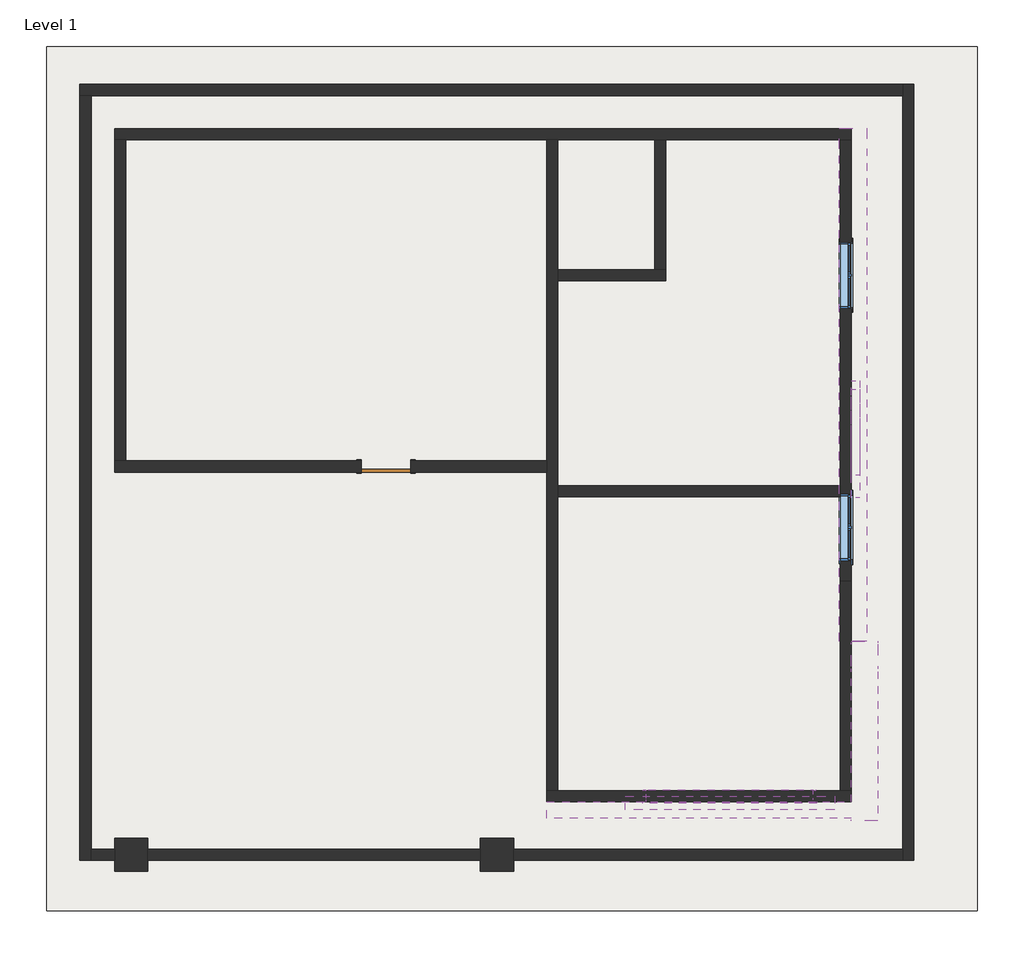
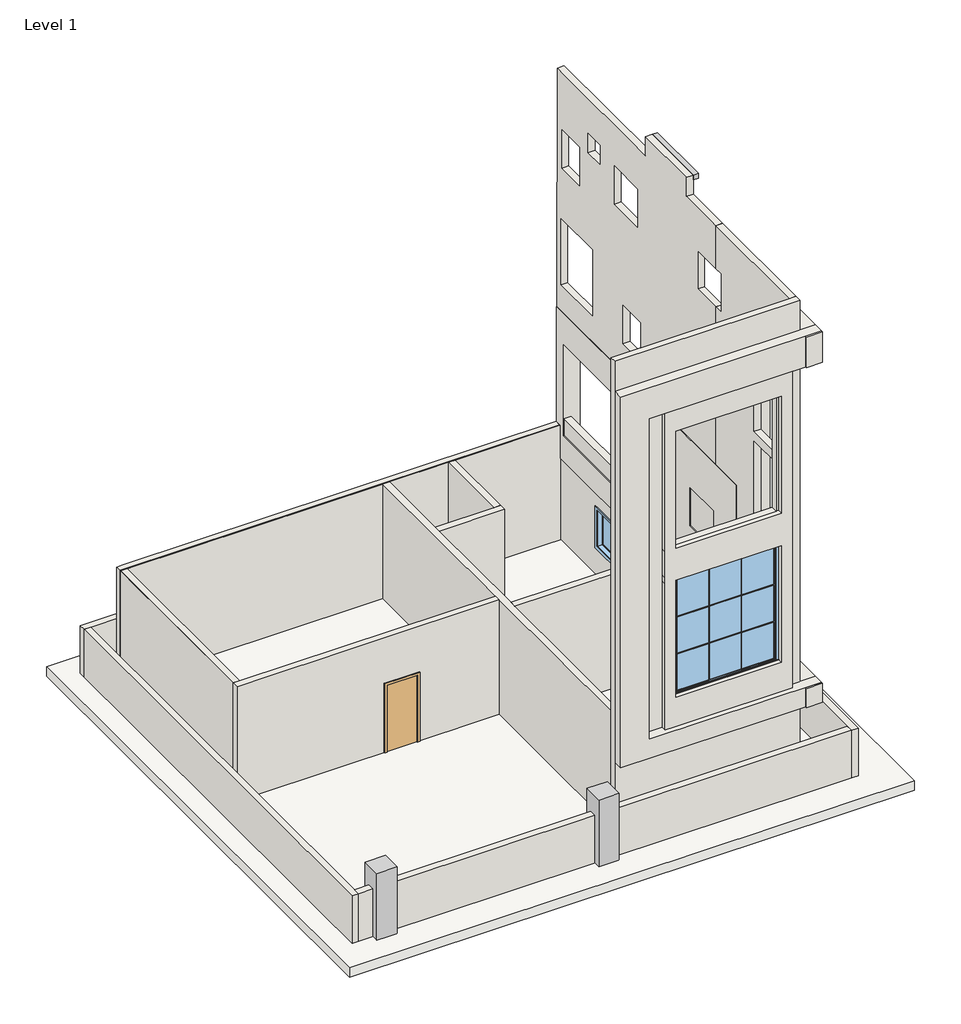
# One storey: 19 walls, 3 windows, 2 columns, 2 proxies, 1 door, 1 slab.
"""IFC4 building model written with IfcOpenShell, lengths in millimetres."""

from ifc_helpers import new_model, si_unit, frame, origin, origin_with_axes, place, context, project, spatial, polyline, outline, extrude, faceted_brep, transform, mapped, element, save
from components import door_54dd4da4, walls_1_walls_1_fa617820, walls_5_walls_5_f65b2cef, walls_7_walls_7_b227ebcc, window_cae7f124, window_0862ab64

model = new_model("IFC4")

# Units and contexts
model_context = context("Model", 3, world=origin())
ifc_project = project(units=[si_unit("LENGTHUNIT", "METRE", prefix="MILLI")], contexts=[model_context])

# Site, building, storey
site = spatial("IfcSite", under=ifc_project)
building = spatial("IfcBuilding", under=site)
storey = spatial("IfcBuildingStorey", under=building, Name="Level 1", Elevation=0.0)

# Proxies
placement = place(None, origin())
element("IfcBuildingElementProxy", 1, Name="Cornice", ObjectType="Cornice", at=placement, inside=storey, context=model_context, shape_type="SweptSolid", body=[
    extrude(outline(polyline([(1662.3254876, 6733.2171591), (1814.7254876, 6733.2171591), (1814.7254876, 4588.9609482), (1662.3254876, 4588.9609482), (1662.3254876, 6733.2171591)])), frame((0.0, 0.0, 15392.4), z_axis=(0.0, 0.0, 1.0), x_axis=(1.0, 0.0, 0.0)), (0.0, 0.0, 1.0), 152.4),
])
element("IfcBuildingElementProxy", 2, Name="Cornice", ObjectType="Cornice", at=placement, inside=storey, context=model_context, shape_type="SweptSolid", body=[
    extrude(outline(polyline([(1662.3254876, 6572.7173646), (1814.7254876, 6572.7173646), (1814.7254876, 4997.9173646), (1662.3254876, 4997.9173646), (1662.3254876, 6572.7173646)])), frame((0.0, 0.0, 12192.0), z_axis=(0.0, 0.0, 1.0), x_axis=(1.0, 0.0, 0.0)), (0.0, 0.0, 1.0), 152.4),
])

# Columns
element("IfcColumn", 3, ObjectType="Rectangular Column : 24\" x 24\"", at=placement, inside=storey, context=model_context, shape_type="Brep", body=[
    faceted_brep([(-11240.8745124, -1652.1419198, 2133.6), (-11850.4745124, -1652.1419198, 2133.6), (-11850.4745124, -2261.7419198, 2133.6), (-11240.8745124, -2261.7419198, 2133.6), (-11240.8745124, -1652.1419198, 0.0), (-11240.8745124, -1855.3419198, 0.0), (-11240.8745124, -2058.5419198, 0.0), (-11240.8745124, -2261.7419198, 0.0), (-11850.4745124, -2261.7419198, 0.0), (-11850.4745124, -2058.5419198, 0.0), (-11850.4745124, -1855.3419198, 0.0), (-11850.4745124, -1652.1419198, 0.0)], [[[0, 1, 2, 3]], [[4, 5, 6, 7, 8, 9, 10, 11]], [[1, 0, 4, 11]], [[2, 1, 11, 10, 9, 8]], [[3, 2, 8, 7]], [[0, 3, 7, 6, 5, 4]]]),
])
element("IfcColumn", 4, ObjectType="Rectangular Column : 24\" x 24\"", at=placement, inside=storey, context=model_context, shape_type="Brep", body=[
    faceted_brep([(-4533.4058988, -1652.1419198, 2133.6), (-5143.0058988, -1652.1419198, 2133.6), (-5143.0058988, -2261.7419198, 2133.6), (-4533.4058988, -2261.7419198, 2133.6), (-4533.4058988, -1652.1419198, 0.0), (-4533.4058988, -1855.3419198, 0.0), (-4533.4058988, -2058.5419198, 0.0), (-4533.4058988, -2261.7419198, 0.0), (-5143.0058988, -2261.7419198, 0.0), (-5143.0058988, -2058.5419198, 0.0), (-5143.0058988, -1855.3419198, 0.0), (-5143.0058988, -1652.1419198, 0.0)], [[[0, 1, 2, 3]], [[4, 5, 6, 7, 8, 9, 10, 11]], [[1, 0, 4, 11]], [[2, 1, 11, 10, 9, 8]], [[3, 2, 8, 7]], [[0, 3, 7, 6, 5, 4]]]),
])

# Door
door_shape = door_54dd4da4(model_context)
element("IfcDoor", 5, ObjectType="Single-Flush : 36\" x 84\"", at=placement, inside=storey, context=model_context, shape_type="MappedRepresentation", body=[
    mapped(door_shape, transform((-6872.0745124, 5160.4609482, 0.0), x_axis=(-1.0, 0.0, 0.0), y_axis=(0.0, -1.0, 0.0), z_axis=(0.0, 0.0, 1.0))),
])

# Slab
element("IfcSlab", 6, ObjectType="Generic - 12\"", at=placement, inside=storey, context=model_context, shape_type="SweptSolid", body=[
    extrude(outline(polyline([(3972.1194136, 12860.9919886), (3972.1194136, -2988.6080114), (-13096.6805864, -2988.6080114), (-13096.6805864, 12860.9919886), (3972.1194136, 12860.9919886)])), frame((0.0, 0.0, -304.8), z_axis=(0.0, 0.0, 1.0), x_axis=(1.0, 0.0, 0.0)), (0.0, 0.0, 1.0), 304.8),
])

# Walls
element("IfcWall", 7, ObjectType="Generic - 8\"", at=placement, inside=storey, context=model_context, shape_type="Brep", body=[
    faceted_brep([(-11850.4745124, 11154.8609482, 0.0), (-11647.2745124, 11154.8609482, 0.0), (-3925.6745124, 11154.8609482, 0.0), (-3722.4745124, 11154.8609482, 0.0), (-1944.4745124, 11154.8609482, 0.0), (-1741.2745124, 11154.8609482, 0.0), (1459.1254876, 11154.8609482, 0.0), (1662.3254876, 11154.8609482, 0.0), (1662.3254876, 11154.8609482, 3657.6), (1459.1254876, 11154.8609482, 3657.6), (1433.7254876, 11154.8609482, 3657.6), (-1741.2745124, 11154.8609482, 3657.6), (-1944.4745124, 11154.8609482, 3657.6), (-3722.4745124, 11154.8609482, 3657.6), (-3925.6745124, 11154.8609482, 3657.6), (-11647.2745124, 11154.8609482, 3657.6), (-11847.2995124, 11154.8609482, 3657.6), (-11850.4745124, 11154.8609482, 3657.6), (-11850.4745124, 11358.0609482, 0.0), (-11850.4745124, 11358.0609482, 3657.6), (-11847.2995124, 11358.0609482, 3657.6), (-11647.2745124, 11358.0609482, 3657.6), (1433.7254876, 11358.0609482, 3657.6), (1459.1254876, 11358.0609482, 3657.6), (1662.3254876, 11358.0609482, 3657.6), (1662.3254876, 11358.0609482, 0.0), (1662.3254876, 11192.9609482, 3657.6), (-11850.4745124, 11192.9609482, 3657.6), (1433.7254876, 11192.9609482, 3657.6), (-11847.2995124, 11192.9609482, 3657.6)], [[[0, 1, 2, 3, 4, 5, 6, 7, 8, 9, 10, 11, 12, 13, 14, 15, 16, 17]], [[18, 19, 20, 21, 22, 23, 24, 25]], [[7, 6, 5, 4, 3, 2, 1, 0, 18, 25]], [[8, 7, 25, 24, 26]], [[0, 17, 27, 19, 18]], [[10, 9, 8, 26, 28]], [[26, 24, 23, 22, 28]], [[17, 16, 29, 27]], [[22, 21, 20, 29, 28]], [[20, 19, 27, 29]], [[16, 15, 14, 13, 12, 11, 10, 28, 29]]]),
])
element("IfcWall", 8, ObjectType="Generic - 8\"", at=placement, inside=storey, context=model_context, shape_type="Brep", body=[
    faceted_brep([(-11850.4745124, 5058.8609482, 0.0), (-7329.2745124, 5058.8609482, 0.0), (-7329.2745124, 5058.8609482, 2133.6), (-6414.8745124, 5058.8609482, 2133.6), (-6414.8745124, 5058.8609482, 0.0), (-3925.6745124, 5058.8609482, 0.0), (-3925.6745124, 5058.8609482, 3657.6), (-11847.2995124, 5058.8609482, 3657.6), (-11850.4745124, 5058.8609482, 3657.6), (-7329.2745124, 5262.0609482, 2133.6), (-7329.2745124, 5262.0609482, 0.0), (-11647.2745124, 5262.0609482, 0.0), (-11850.4745124, 5262.0609482, 0.0), (-11850.4745124, 5262.0609482, 3657.6), (-11847.2995124, 5262.0609482, 3657.6), (-11647.2745124, 5262.0609482, 3657.6), (-3925.6745124, 5262.0609482, 3657.6), (-3925.6745124, 5262.0609482, 0.0), (-6414.8745124, 5262.0609482, 0.0), (-6414.8745124, 5262.0609482, 2133.6)], [[[0, 1, 2, 3, 4, 5, 6, 7, 8]], [[9, 10, 11, 12, 13, 14, 15, 16, 17, 18, 19]], [[18, 17, 5, 4]], [[12, 11, 10, 1, 0]], [[6, 5, 17, 16]], [[0, 8, 13, 12]], [[8, 7, 14, 13]], [[7, 6, 16, 15, 14]], [[2, 1, 10, 9]], [[3, 2, 9, 19]], [[4, 3, 19, 18]]]),
])
element("IfcWall", 9, ObjectType="Generic - 8\"", at=placement, inside=storey, context=model_context, shape_type="Brep", body=[
    faceted_brep([(-3925.6745124, 11154.8609482, 0.0), (-3925.6745124, 5262.0609482, 0.0), (-3925.6745124, 5058.8609482, 0.0), (-3925.6745124, -783.1390518, 0.0), (-3925.6745124, -783.1390518, 3657.6), (-3925.6745124, 1858.4609482, 3657.6), (-3925.6745124, 5058.8609482, 3657.6), (-3925.6745124, 5262.0609482, 3657.6), (-3925.6745124, 11154.8609482, 3657.6), (-3722.4745124, 11154.8609482, 0.0), (-3722.4745124, 11154.8609482, 3657.6), (-3722.4745124, 8767.2609482, 3657.6), (-3722.4745124, 8564.0609482, 3657.6), (-3722.4745124, 4804.8609482, 3657.6), (-3722.4745124, 4601.6609482, 3657.6), (-3722.4745124, 1858.4609482, 3657.6), (-3722.4745124, -783.1390518, 3657.6), (-3722.4745124, -783.1390518, 0.0), (-3722.4745124, 4601.6609482, 0.0), (-3722.4745124, 4804.8609482, 0.0), (-3722.4745124, 8564.0609482, 0.0), (-3722.4745124, 8767.2609482, 0.0)], [[[0, 1, 2, 3, 4, 5, 6, 7, 8]], [[9, 10, 11, 12, 13, 14, 15, 16, 17, 18, 19, 20, 21]], [[3, 2, 1, 0, 9, 21, 20, 19, 18, 17]], [[8, 7, 6, 5, 4, 16, 15, 14, 13, 12, 11, 10]], [[4, 3, 17, 16]], [[0, 8, 10, 9]]]),
])
element("IfcWall", 10, ObjectType="Generic - 8\"", at=placement, inside=storey, context=model_context, shape_type="SweptSolid", body=[
    extrude(outline(polyline([(3657.6, -11850.4745124), (0.0, -11850.4745124), (0.0, -11647.2745124), (3657.6, -11647.2745124), (3657.6, -11847.2995124), (3657.6, -11850.4745124)])), frame((0.0, 5262.0609482, 0.0), z_axis=(0.0, 1.0, 0.0), x_axis=(0.0, 0.0, 1.0)), (0.0, 0.0, 1.0), 5892.8),
])
element("IfcWall", 11, ObjectType="Generic - 8\"", at=placement, inside=storey, context=model_context, shape_type="Brep", body=[
    faceted_brep([(-3925.6745124, -986.3390518, 14935.2), (-3925.6745124, -986.3390518, 0.0), (1662.3254876, -986.3390518, 0.0), (1662.3254876, -986.3390518, 14935.2), (-2096.8745124, -986.3390518, 12107.4316285), (951.1254876, -986.3390518, 12107.4316285), (951.1254876, -986.3390518, 8449.8316285), (-2096.8745124, -986.3390518, 8449.8316285), (-2096.8745124, -986.3390518, 7347.484706), (951.1254876, -986.3390518, 7347.484706), (951.1254876, -986.3390518, 3689.884706), (-2096.8745124, -986.3390518, 3689.884706), (-3925.6745124, -783.1390518, 0.0), (-3925.6745124, -783.1390518, 3657.6), (-3925.6745124, -783.1390518, 10972.8), (-3925.6745124, -783.1390518, 14935.2), (1459.1254876, -783.1390518, 14935.2), (1662.3254876, -783.1390518, 14935.2), (1662.3254876, -783.1390518, 0.0), (1459.1254876, -783.1390518, 0.0), (-3722.4745124, -783.1390518, 0.0), (-2096.8745124, -783.1390518, 12107.4316285), (-2096.8745124, -783.1390518, 8449.8316285), (951.1254876, -783.1390518, 8449.8316285), (951.1254876, -783.1390518, 12107.4316285), (-2096.8745124, -783.1390518, 7347.484706), (-2096.8745124, -783.1390518, 3689.884706), (951.1254876, -783.1390518, 3689.884706), (951.1254876, -783.1390518, 7347.484706)], [[[0, 1, 2, 3], [4, 5, 6, 7], [8, 9, 10, 11]], [[12, 13, 14, 15, 16, 17, 18, 19, 20], [21, 22, 23, 24], [25, 26, 27, 28]], [[2, 1, 12, 20, 19, 18]], [[0, 3, 17, 16, 15]], [[3, 2, 18, 17]], [[0, 15, 14, 13, 12, 1]], [[22, 21, 4, 7]], [[23, 22, 7, 6]], [[24, 23, 6, 5]], [[21, 24, 5, 4]], [[26, 25, 8, 11]], [[27, 26, 11, 10]], [[28, 27, 10, 9]], [[25, 28, 9, 8]]]),
])
element("IfcWall", 12, ObjectType="Generic - 8\"", at=placement, inside=storey, context=model_context, shape_type="SweptSolid", body=[
    extrude(outline(polyline([(3052.2609482, 0.0), (-783.1390518, 0.0), (-783.1390518, 14935.2), (3052.2609482, 14935.2), (3052.2609482, 13563.6), (2772.8609482, 13563.6), (2772.8609482, 12344.4), (3052.2609482, 12344.4), (3052.2609482, 0.0)]), holes=[polyline([(1055.2332725, 9576.1019988), (1055.2332725, 12522.5019988), (-163.9667275, 12522.5019988), (-163.9667275, 9576.1019988), (1055.2332725, 9576.1019988)]), polyline([(1055.2332725, 6324.9019988), (1055.2332725, 9271.3019988), (-163.9667275, 9271.3019988), (-163.9667275, 6324.9019988), (1055.2332725, 6324.9019988)]), polyline([(1055.2332725, 3022.9019988), (1055.2332725, 5969.3019988), (-163.9667275, 5969.3019988), (-163.9667275, 3022.9019988), (1055.2332725, 3022.9019988)])]), frame((1459.1254876, 0.0, 0.0), z_axis=(1.0, 0.0, 0.0), x_axis=(0.0, 1.0, 0.0)), (0.0, 0.0, 1.0), 203.2),
])
element("IfcWall", 13, ObjectType="Generic - 8\"", at=placement, inside=storey, context=model_context, shape_type="Brep", body=[
    faceted_brep([(1459.1254876, 11154.8609482, 0.0), (1459.1254876, 4804.8609482, 0.0), (1459.1254876, 4601.6609482, 0.0), (1459.1254876, 3052.2609482, 0.0), (1459.1254876, 3052.2609482, 12344.4), (1459.1254876, 3992.0609482, 12344.4), (1459.1254876, 3992.0609482, 13563.6), (1459.1254876, 3052.2609482, 13563.6), (1459.1254876, 3052.2609482, 14935.2), (1459.1254876, 4588.9609482, 14935.2), (1459.1254876, 4588.9609482, 15544.8), (1459.1254876, 6733.2171591, 15544.8), (1459.1254876, 6733.2171591, 14935.2), (1459.1254876, 11142.1609482, 14935.2), (1459.1254876, 11345.3609482, 14935.2), (1459.1254876, 11345.3609482, 11277.6), (1459.1254876, 11358.0609482, 11277.6), (1459.1254876, 11358.0609482, 7623.0321664), (1459.1254876, 11358.0609482, 7315.2), (1459.1254876, 11358.0609482, 3657.6), (1459.1254876, 11154.8609482, 3657.6), (1459.1254876, 9732.4609482, 13828.4684583), (1459.1254876, 9122.8609482, 13828.4684583), (1459.1254876, 9122.8609482, 13218.8684583), (1459.1254876, 9732.4609482, 13218.8684583), (1459.1254876, 7141.6609482, 13622.4204192), (1459.1254876, 7141.6609482, 12403.2204192), (1459.1254876, 8360.8609482, 12403.2204192), (1459.1254876, 8360.8609482, 13622.4204192), (1459.1254876, 10189.6609482, 13106.4), (1459.1254876, 10189.6609482, 11887.2), (1459.1254876, 11104.0609482, 11887.2), (1459.1254876, 11104.0609482, 13106.4), (1459.1254876, 4855.6609482, 9448.8), (1459.1254876, 3941.2609482, 9448.8), (1459.1254876, 3941.2609482, 8229.6), (1459.1254876, 4855.6609482, 8229.6), (1459.1254876, 7903.6609482, 9448.8), (1459.1254876, 6989.2609482, 9448.8), (1459.1254876, 6989.2609482, 8229.6), (1459.1254876, 7903.6609482, 8229.6), (1459.1254876, 11154.8609482, 10244.4876686), (1459.1254876, 9518.25414, 10244.4876686), (1459.1254876, 9518.25414, 8130.9177257), (1459.1254876, 11154.8609482, 8130.9177257), (1459.1254876, 3433.2609482, 2133.6), (1459.1254876, 3433.2609482, 914.4), (1459.1254876, 4652.4609482, 914.4), (1459.1254876, 4652.4609482, 2133.6), (1459.1254876, 8056.0609482, 2133.6), (1459.1254876, 8056.0609482, 914.4), (1459.1254876, 9275.2609482, 914.4), (1459.1254876, 9275.2609482, 2133.6), (1459.1254876, 10990.2518123, 6324.9019988), (1459.1254876, 7724.717248, 6324.9019988), (1459.1254876, 7724.717248, 3962.4), (1459.1254876, 10990.2518123, 3962.4), (1459.1254876, 7185.0917513, 6324.9019988), (1459.1254876, 5580.0518123, 6324.9019988), (1459.1254876, 5580.0518123, 3962.4), (1459.1254876, 7185.0917513, 3962.4), (1662.3254876, 3052.2609482, 0.0), (1662.3254876, 11154.8609482, 0.0), (1662.3254876, 11154.8609482, 3657.6), (1662.3254876, 11358.0609482, 3657.6), (1662.3254876, 11358.0609482, 11277.6), (1662.3254876, 11345.3609482, 11277.6), (1662.3254876, 11345.3609482, 14935.2), (1662.3254876, 6733.2171591, 14935.2), (1662.3254876, 6733.2171591, 15544.8), (1662.3254876, 4588.9609482, 15544.8), (1662.3254876, 4588.9609482, 14935.2), (1662.3254876, 3052.2609482, 14935.2), (1662.3254876, 3052.2609482, 13563.6), (1662.3254876, 3992.0609482, 13563.6), (1662.3254876, 3992.0609482, 12344.4), (1662.3254876, 3052.2609482, 12344.4), (1662.3254876, 9732.4609482, 13828.4684583), (1662.3254876, 9732.4609482, 13218.8684583), (1662.3254876, 9122.8609482, 13218.8684583), (1662.3254876, 9122.8609482, 13828.4684583), (1662.3254876, 7141.6609482, 13622.4204192), (1662.3254876, 8360.8609482, 13622.4204192), (1662.3254876, 8360.8609482, 12403.2204192), (1662.3254876, 7141.6609482, 12403.2204192), (1662.3254876, 10189.6609482, 13106.4), (1662.3254876, 11104.0609482, 13106.4), (1662.3254876, 11104.0609482, 11887.2), (1662.3254876, 10189.6609482, 11887.2), (1662.3254876, 4855.6609482, 9448.8), (1662.3254876, 4855.6609482, 8229.6), (1662.3254876, 3941.2609482, 8229.6), (1662.3254876, 3941.2609482, 9448.8), (1662.3254876, 7903.6609482, 9448.8), (1662.3254876, 7903.6609482, 8229.6), (1662.3254876, 6989.2609482, 8229.6), (1662.3254876, 6989.2609482, 9448.8), (1662.3254876, 9518.25414, 10244.4876686), (1662.3254876, 11154.8609482, 10244.4876686), (1662.3254876, 11154.8609482, 8130.9177257), (1662.3254876, 9518.25414, 8130.9177257), (1662.3254876, 3433.2609482, 2133.6), (1662.3254876, 4652.4609482, 2133.6), (1662.3254876, 4652.4609482, 914.4), (1662.3254876, 3433.2609482, 914.4), (1662.3254876, 8056.0609482, 2133.6), (1662.3254876, 9275.2609482, 2133.6), (1662.3254876, 9275.2609482, 914.4), (1662.3254876, 8056.0609482, 914.4), (1662.3254876, 7724.717248, 6324.9019988), (1662.3254876, 10990.2518123, 6324.9019988), (1662.3254876, 10990.2518123, 3962.4), (1662.3254876, 7724.717248, 3962.4), (1662.3254876, 5580.0518123, 6324.9019988), (1662.3254876, 7185.0917513, 6324.9019988), (1662.3254876, 7185.0917513, 3962.4), (1662.3254876, 5580.0518123, 3962.4)], [[[0, 1, 2, 3, 4, 5, 6, 7, 8, 9, 10, 11, 12, 13, 14, 15, 16, 17, 18, 19, 20], [21, 22, 23, 24], [25, 26, 27, 28], [29, 30, 31, 32], [33, 34, 35, 36], [37, 38, 39, 40], [41, 42, 43, 44], [45, 46, 47, 48], [49, 50, 51, 52], [53, 54, 55, 56], [57, 58, 59, 60]], [[61, 62, 63, 64, 65, 66, 67, 68, 69, 70, 71, 72, 73, 74, 75, 76], [77, 78, 79, 80], [81, 82, 83, 84], [85, 86, 87, 88], [89, 90, 91, 92], [93, 94, 95, 96], [97, 98, 99, 100], [101, 102, 103, 104], [105, 106, 107, 108], [109, 110, 111, 112], [113, 114, 115, 116]], [[0, 20, 63, 62]], [[19, 18, 17, 16, 65, 64]], [[15, 14, 67, 66]], [[3, 2, 1, 0, 62, 61]], [[3, 61, 76, 4]], [[72, 8, 7, 73]], [[64, 63, 20, 19]], [[66, 65, 16, 15]], [[9, 8, 72, 71]], [[10, 9, 71, 70]], [[11, 10, 70, 69]], [[12, 11, 69, 68]], [[14, 13, 12, 68, 67]], [[78, 77, 21, 24]], [[79, 78, 24, 23]], [[80, 79, 23, 22]], [[77, 80, 22, 21]], [[75, 5, 4, 76]], [[5, 75, 74, 6]], [[6, 74, 73, 7]], [[26, 25, 81, 84]], [[27, 26, 84, 83]], [[28, 27, 83, 82]], [[25, 28, 82, 81]], [[30, 29, 85, 88]], [[31, 30, 88, 87]], [[32, 31, 87, 86]], [[29, 32, 86, 85]], [[90, 89, 33, 36]], [[91, 90, 36, 35]], [[92, 91, 35, 34]], [[89, 92, 34, 33]], [[94, 93, 37, 40]], [[95, 94, 40, 39]], [[96, 95, 39, 38]], [[93, 96, 38, 37]], [[42, 41, 98, 97]], [[43, 42, 97, 100]], [[44, 43, 100, 99]], [[41, 44, 99, 98]], [[46, 45, 101, 104]], [[47, 46, 104, 103]], [[48, 47, 103, 102]], [[45, 48, 102, 101]], [[50, 49, 105, 108]], [[51, 50, 108, 107]], [[52, 51, 107, 106]], [[49, 52, 106, 105]], [[54, 53, 110, 109]], [[55, 54, 109, 112]], [[56, 55, 112, 111]], [[53, 56, 111, 110]], [[58, 57, 114, 113]], [[59, 58, 113, 116]], [[60, 59, 116, 115]], [[57, 60, 115, 114]]]),
])
element("IfcWall", 14, ObjectType="Generic - 8\"", at=placement, inside=storey, context=model_context, shape_type="SweptSolid", body=[
    extrude(outline(polyline([(1459.1254876, 4601.6609482), (-3722.4745124, 4601.6609482), (-3722.4745124, 4804.8609482), (1459.1254876, 4804.8609482), (1459.1254876, 4601.6609482)])), origin_with_axes(), (0.0, 0.0, 1.0), 3657.6),
])
element("IfcWall", 15, ObjectType="Generic - 8\"", at=placement, inside=storey, context=model_context, shape_type="Brep", body=[
    faceted_brep([(-3722.4745124, 8564.0609482, 0.0), (-1741.2745124, 8564.0609482, 0.0), (-1741.2745124, 8564.0609482, 3657.6), (-3722.4745124, 8564.0609482, 3657.6), (-3722.4745124, 8767.2609482, 0.0), (-3722.4745124, 8767.2609482, 3657.6), (-1944.4745124, 8767.2609482, 3657.6), (-1741.2745124, 8767.2609482, 3657.6), (-1741.2745124, 8767.2609482, 0.0), (-1944.4745124, 8767.2609482, 0.0)], [[[0, 1, 2, 3]], [[4, 5, 6, 7, 8, 9]], [[1, 0, 4, 9, 8]], [[3, 2, 7, 6, 5]], [[0, 3, 5, 4]], [[2, 1, 8, 7]]]),
])
element("IfcWall", 16, ObjectType="Generic - 8\"", at=placement, inside=storey, context=model_context, shape_type="SweptSolid", body=[
    extrude(outline(polyline([(-1741.2745124, 11154.8609482), (-1741.2745124, 8767.2609482), (-1944.4745124, 8767.2609482), (-1944.4745124, 11154.8609482), (-1741.2745124, 11154.8609482)])), origin_with_axes(), (0.0, 0.0, 1.0), 3657.6),
])
element("IfcWall", 17, ObjectType="Generic - 8\"", at=placement, inside=storey, context=model_context, shape_type="Brep", body=[
    faceted_brep([(-12483.6058988, 11962.2580802, 0.0), (-12280.4058988, 11962.2580802, 0.0), (2603.9941012, 11962.2580802, 0.0), (2603.9941012, 11962.2580802, 1524.0), (-12280.4058988, 11962.2580802, 1524.0), (-12483.6058988, 11962.2580802, 1524.0), (-12483.6058988, 12165.4580802, 0.0), (-12483.6058988, 12165.4580802, 1524.0), (2603.9941012, 12165.4580802, 1524.0), (2603.9941012, 12165.4580802, 0.0)], [[[0, 1, 2, 3, 4, 5]], [[6, 7, 8, 9]], [[2, 1, 0, 6, 9]], [[5, 4, 3, 8, 7]], [[0, 5, 7, 6]], [[3, 2, 9, 8]]]),
])
element("IfcWall", 18, ObjectType="Generic - 8\"", at=placement, inside=storey, context=model_context, shape_type="Brep", body=[
    faceted_brep([(-12280.4058988, -2058.5419198, 0.0), (-12280.4058988, -1855.3419198, 0.0), (-12280.4058988, 11962.2580802, 0.0), (-12280.4058988, 11962.2580802, 1524.0), (-12280.4058988, -1855.3419198, 1524.0), (-12280.4058988, -2058.5419198, 1524.0), (-12483.6058988, -2058.5419198, 0.0), (-12483.6058988, -2058.5419198, 1524.0), (-12483.6058988, 11962.2580802, 1524.0), (-12483.6058988, 11962.2580802, 0.0)], [[[0, 1, 2, 3, 4, 5]], [[6, 7, 8, 9]], [[2, 1, 0, 6, 9]], [[5, 4, 3, 8, 7]], [[3, 2, 9, 8]], [[0, 5, 7, 6]]]),
])
element("IfcWall", 19, ObjectType="Generic - 8\"", at=placement, inside=storey, context=model_context, shape_type="SweptSolid", body=[
    extrude(outline(polyline([(-11240.8745124, -1855.3419198), (-5143.0058988, -1855.3419198), (-5143.0058988, -2058.5419198), (-11240.8745124, -2058.5419198), (-11240.8745124, -1855.3419198)])), origin_with_axes(), (0.0, 0.0, 1.0), 1524.0),
])
element("IfcWall", 20, ObjectType="Generic - 8\"", at=placement, inside=storey, context=model_context, shape_type="Brep", body=[
    faceted_brep([(2603.9941012, 12165.4580802, 0.0), (2603.9941012, 11962.2580802, 0.0), (2603.9941012, -1855.3419198, 0.0), (2603.9941012, -2058.5419198, 0.0), (2603.9941012, -2058.5419198, 1524.0), (2603.9941012, -1855.3419198, 1524.0), (2603.9941012, 11962.2580802, 1524.0), (2603.9941012, 12165.4580802, 1524.0), (2807.1941012, 12165.4580802, 0.0), (2807.1941012, 12165.4580802, 1524.0), (2807.1941012, -2058.5419198, 1524.0), (2807.1941012, -2058.5419198, 0.0)], [[[0, 1, 2, 3, 4, 5, 6, 7]], [[8, 9, 10, 11]], [[3, 2, 1, 0, 8, 11]], [[7, 6, 5, 4, 10, 9]], [[0, 7, 9, 8]], [[4, 3, 11, 10]]]),
])
element("IfcWall", 21, ObjectType="Generic - 8\"", at=placement, inside=storey, context=model_context, shape_type="SweptSolid", body=[
    extrude(outline(polyline([(-11850.4745124, -2058.5419198), (-12280.4058988, -2058.5419198), (-12280.4058988, -1855.3419198), (-11850.4745124, -1855.3419198), (-11850.4745124, -2058.5419198)])), origin_with_axes(), (0.0, 0.0, 1.0), 1524.0),
])
element("IfcWall", 22, ObjectType="Generic - 8\"", at=placement, inside=storey, context=model_context, shape_type="SweptSolid", body=[
    extrude(outline(polyline([(2603.9941012, -2058.5419198), (-4533.4058988, -2058.5419198), (-4533.4058988, -1855.3419198), (2603.9941012, -1855.3419198), (2603.9941012, -2058.5419198)])), origin_with_axes(), (0.0, 0.0, 1.0), 1524.0),
])
walls_1_walls_1_shape = walls_1_walls_1_fa617820(model_context)
element("IfcWall", 23, ObjectType="Walls 1 : Walls 1", at=placement, inside=storey, context=model_context, shape_type="MappedRepresentation", body=[
    mapped(walls_1_walls_1_shape, transform((0.0, 0.0, 0.0), x_axis=(1.0, 0.0, 0.0), y_axis=(0.0, 1.0, 0.0), z_axis=(0.0, 0.0, 1.0))),
])
walls_5_walls_5_shape = walls_5_walls_5_f65b2cef(model_context)
element("IfcWall", 24, ObjectType="Walls 5 : Walls 5", at=placement, inside=storey, context=model_context, shape_type="MappedRepresentation", body=[
    mapped(walls_5_walls_5_shape, transform((0.0, 0.0, 0.0), x_axis=(1.0, 0.0, 0.0), y_axis=(0.0, 1.0, 0.0), z_axis=(0.0, 0.0, 1.0))),
])
walls_7_walls_7_shape = walls_7_walls_7_b227ebcc(model_context)
element("IfcWall", 25, ObjectType="Walls 7 : Walls 7", at=placement, inside=storey, context=model_context, shape_type="MappedRepresentation", body=[
    mapped(walls_7_walls_7_shape, transform((0.0, 0.0, 0.0), x_axis=(1.0, 0.0, 0.0), y_axis=(0.0, 1.0, 0.0), z_axis=(0.0, 0.0, 1.0))),
])

# Windows
window_shape = window_cae7f124(model_context)
element("IfcWindow", 26, ObjectType="Casement 3x3 with Trim : 120\" x 144\"", at=placement, inside=storey, context=model_context, shape_type="MappedRepresentation", body=[
    mapped(window_shape, transform((-572.8745124, -884.7390518, -1796.515294), x_axis=(-1.0, 0.0, 0.0), y_axis=(0.0, -1.0, 0.0), z_axis=(0.0, 0.0, 1.0))),
])
window_2_shape = window_0862ab64(model_context)
element("IfcWindow", 27, ObjectType="Casement Dbl with Trim : 48\" x 48\"", at=placement, inside=storey, context=model_context, shape_type="MappedRepresentation", body=[
    mapped(window_2_shape, transform((1541.6754876, 4042.8609482, 0.0), x_axis=(0.0, -1.0, 0.0), y_axis=(1.0, 0.0, 0.0), z_axis=(0.0, 0.0, 1.0))),
])
element("IfcWindow", 28, ObjectType="Casement Dbl with Trim : 48\" x 48\"", at=placement, inside=storey, context=model_context, shape_type="MappedRepresentation", body=[
    mapped(window_2_shape, transform((1541.6754876, 8665.6609482, 0.0), x_axis=(0.0, -1.0, 0.0), y_axis=(1.0, 0.0, 0.0), z_axis=(0.0, 0.0, 1.0))),
])

save(model, "model.ifc")

# Revit data of these elements
# Type "Rectangular Column : 24\" x 24\""
#   Assembly Code = "B1010200"
#   Depth = 2' - 0"
#   Offset Base = 0' - 0"
#   Offset Top = 0' - 0"
#   Width = 2' - 0"
#   Material = none
# Type "Single-Flush : 36\" x 84\""
#   Type Mark = "1"
#   Construction Type Id = "MDOOR"
#   Assembly Code = "C1020"
#   Analytic Construction = "Metal"
#   Thickness = 0' - 2"
#   Heat Transfer Coefficient (U) = 0.651978 BTU/(h·ft²·°F)
#   Height = 7' - 0"
#   Trim Projection Ext = 0' - 1"
#   Trim Projection Int = 0' - 1"
#   Trim Width = 0' - 3"
#   Width = 3' - 0"
#   Define Thermal Properties by = 1
#   Door Material = Door - Panel
#   Frame Material = Door - Frame
#   Visual Light Transmittance = 0
#   Solar Heat Gain Coefficient = 0
#   Function = (empty or 0)
#   Wall Closure = (empty or 0)
# Type "Generic - 12\""
#   Assembly Code = "B1010"
#   Function = 0
#   Layers, outside or top first: 1' - 0" no material (function 1)
# Type "Generic - 8\""
#   Assembly Code = "B2010"
#   Layers, outside or top first: 0' - 8" no material (function 1)
# Type "Casement 3x3 with Trim : 120\" x 144\""
#   Type Mark = "10"
#   Construction Type Id = "GSP4R"
#   Assembly Code = "B2020100"
#   Analytic Construction = "1/8 in Pilkington single glazing"
#   Visual Light Transmittance = 0.9
#   Solar Heat Gain Coefficient = 0.78
#   Heat Transfer Coefficient (U) = 0.6496 BTU/(h·ft²·°F)
#   Height = 12' - 0"
#   Default Sill Height = 18' - 0"
#   Trim Projection - Ext. = 0' - 0 1/2"
#   Trim Projection - Int. = 0' - 0 3/4"
#   Trim Width - Exterior = 0' - 3 1/2"
#   Trim Width - Interior = 0' - 3 1/2"
#   Width = 10' - 0"
#   Window Inset = 0' - 0 3/4"
#   Define Thermal Properties by = 1
#   Glass Pane Material = Glass
#   Sash Material = Sash
#   Trim Exterior Material = Trim
#   Trim Interior Material = Trim
#   Wall Closure = (empty or 0)
# Type "Casement Dbl with Trim : 48\" x 48\""
#   Type Mark = "13"
#   Construction Type Id = "GSP4R"
#   Assembly Code = "B2020100"
#   Analytic Construction = "1/8 in Pilkington single glazing"
#   Visual Light Transmittance = 0.9
#   Solar Heat Gain Coefficient = 0.78
#   Heat Transfer Coefficient (U) = 0.6496 BTU/(h·ft²·°F)
#   Height = 4' - 0"
#   Default Sill Height = 3' - 0"
#   Trim Projection - Ext. = 0' - 0 1/2"
#   Trim Projection - Int. = 0' - 0 3/4"
#   Trim Width - Exterior = 0' - 3 1/2"
#   Trim Width - Interior = 0' - 3 1/2"
#   Width = 4' - 0"
#   Window Inset = 0' - 0 3/4"
#   Define Thermal Properties by = 1
#   Glass Pane Material = Glass
#   Sash Material = Sash
#   Trim Exterior Material = Trim
#   Trim Interior Material = Trim
#   Wall Closure = (empty or 0)
# Elements 1, 2 (IfcBuildingElementProxy, "Cornice")
#   Phase Created = New Construction
#   Materials on its faces: "Default Wall"
# Elements 3, 4 (IfcColumn, "Rectangular Column : 24\" x 24\"")
#   Phase Created = New Construction
#   Materials on its faces: "Default Wall"
# Element 5 (IfcDoor, "Single-Flush : 36\" x 84\"")
#   Phase Created = New Construction
#   Materials on its faces: "Door - Frame", "Door - Panel"
# Element 6 (IfcSlab, "Generic - 12\"")
#   Height Offset From Level = 0' - 0"
#   Phase Created = New Construction
#   Materials on its faces: "Default Floor"
# Elements 7, 8, 9, 10, 14, 15, 16 (IfcWall, "Generic - 8\"")
#   Top Offset = 0' - 0"
#   Base Offset = 0' - 0"
#   Unconnected Height = 12' - 0"
#   wall height = 12' - 0"
#   Phase Created = New Construction
#   Base Constraint = Level 1
#   Materials on its faces: "Default Wall"
# Elements 11, 12, 13 (IfcWall, "Generic - 8\"")
#   Top Offset = 0' - 0"
#   Base Offset = 0' - 0"
#   Unconnected Height = 49' - 0"
#   wall height = 49' - 0"
#   Phase Created = New Construction
#   Base Constraint = Level 1
#   Materials on its faces: "Default Wall"
# Elements 17, 18, 19, 20, 21, 22 (IfcWall, "Generic - 8\"")
#   Top Offset = 0' - 0"
#   Base Offset = 0' - 0"
#   Unconnected Height = 5' - 0"
#   wall height = 5' - 0"
#   Phase Created = New Construction
#   Base Constraint = Level 1
#   Materials on its faces: "Default Wall"
# Element 23 (IfcWall, "Walls 1 : Walls 1")
#   Phase Created = New Construction
#   Materials on its faces: "Default Wall"
# Element 24 (IfcWall, "Walls 5 : Walls 5")
#   Phase Created = New Construction
#   Materials on its faces: "Default Wall"
# Element 25 (IfcWall, "Walls 7 : Walls 7")
#   Phase Created = New Construction
#   Materials on its faces: "Default Wall"
# Element 26 (IfcWindow, "Casement 3x3 with Trim : 120\" x 144\"")
#   Mark = "2"
#   Phase Created = New Construction
#   Materials on its faces: "Sash", "Glass", "Trim"
# Element 27 (IfcWindow, "Casement Dbl with Trim : 48\" x 48\"")
#   Mark = "13"
#   Phase Created = New Construction
#   Materials on its faces: "Sash", "Trim", "Glass"
# Element 28 (IfcWindow, "Casement Dbl with Trim : 48\" x 48\"")
#   Mark = "14"
#   Phase Created = New Construction
#   Materials on its faces: "Sash", "Trim", "Glass"
# Materials
#   "Door - Panel": class "Wood", colour RGB 210 159 95, transparency 0
#   "Door - Frame": colour RGB 118 70 51, transparency 0
#   "Glass": class "Glass", colour RGB 0 128 192, transparency 0.75, Description = "Soda Lime Glass", Cost = 0
#   "Sash": class "Wood", colour RGB 224 178 126, transparency 0
#   "Trim": class "Wood", colour RGB 224 178 126, transparency 0
#   "Default Wall": colour RGB 128 128 128, transparency 0
#   "Default Floor": colour RGB 128 128 128, transparency 0
